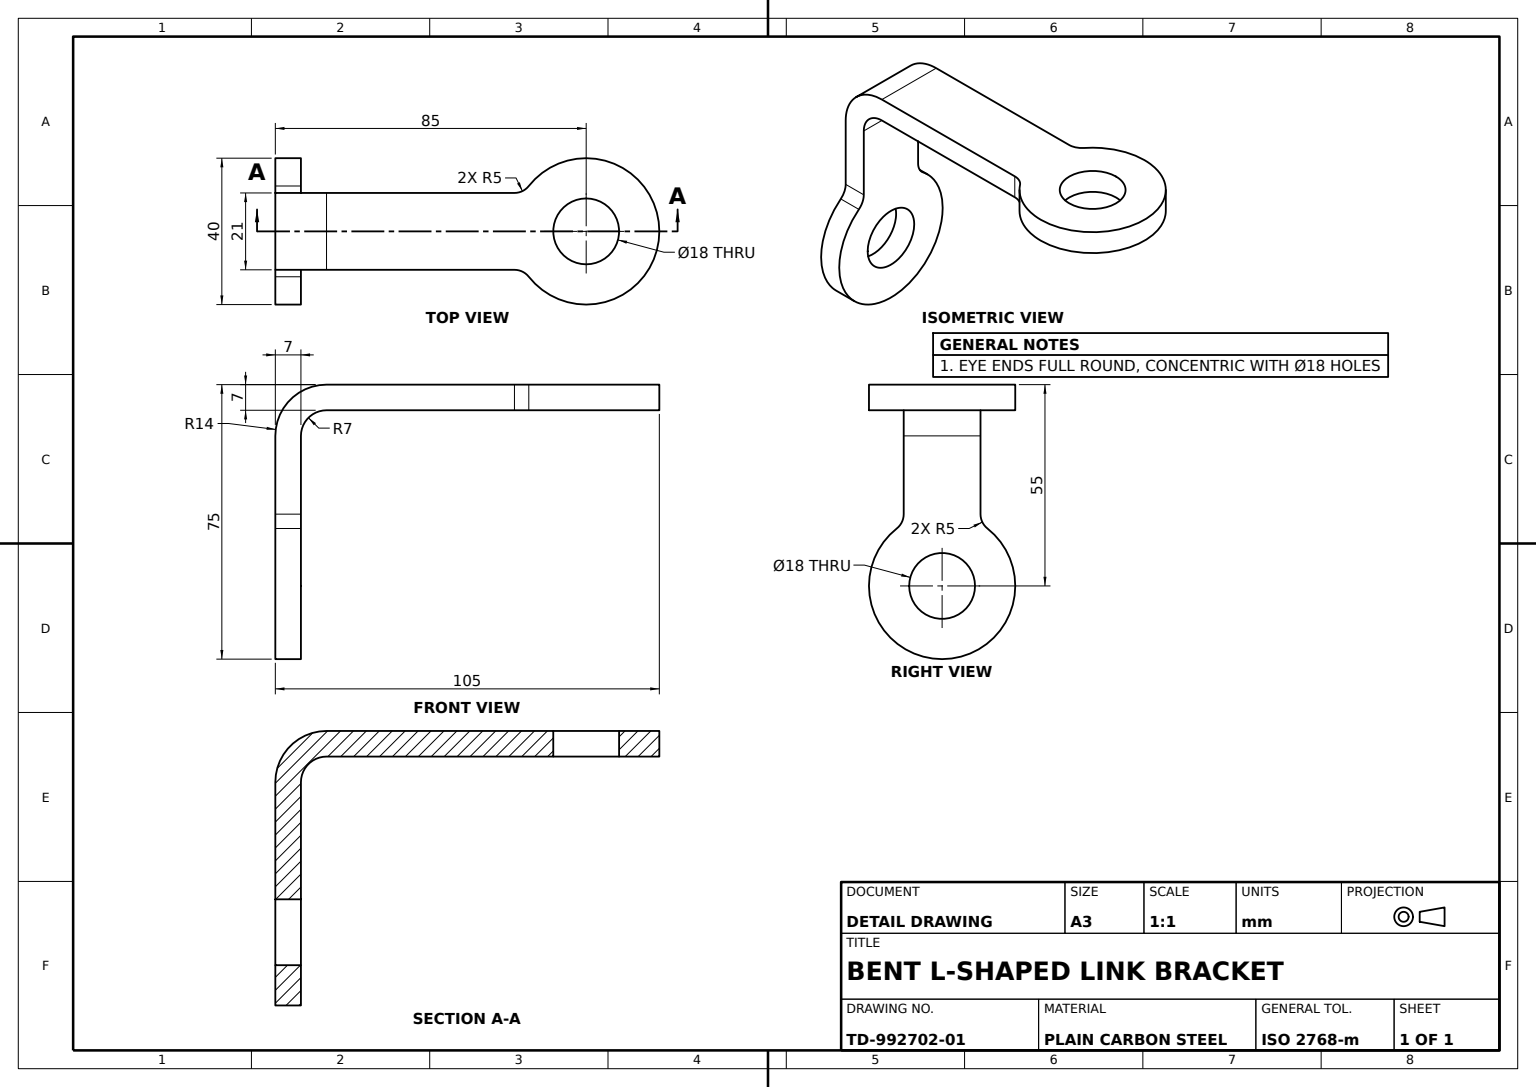
from build123d import *

# Parameters (mm, degrees)
HORIZONTAL_ARM_PROFILE_R    = 9
HORIZONTAL_ARM_7MM_DEPTH    = 7
VERTICAL_ARM_PROFILE_R      = 9
VERTICAL_ARM_7MM_DEPTH      = 7
BEND_FILLET_R5_R            = 5
HORIZONTAL_ARM_FILLET_R14_R = 14
BEND_FILLET_R7_R            = 7


with BuildPart() as part:
    # Horizontal Arm Profile → Horizontal Arm 7mm (new body)
    with BuildSketch(Plane(origin=(0, 0, 0), x_dir=(1, 0, 0), z_dir=(0, 1, 0))):
        with BuildLine():
            Line((-17.022044531, 10.5), (-85, 10.5))
            Line((-85, 10.5), (-85, -10.5))
            Line((-85, -10.5), (-17.022044531, -10.5))
            ThreePointArc((-17.022044531, -10.5), (20, 0), (-17.022044531, 10.5))
        make_face()
        with Locations(Location((0, 0, 0), (0, 0, 270))):
            Circle(HORIZONTAL_ARM_PROFILE_R, mode=Mode.SUBTRACT)
    extrude(amount=-HORIZONTAL_ARM_7MM_DEPTH)

    # Vertical Arm Profile → Vertical Arm 7mm (add)
    with BuildSketch(Plane(origin=(-85, 0, 0), x_dir=(0, 0, -1), z_dir=(1, 0, 0))):
        with BuildLine():
            Line((-10.5, 0), (-10.5, -37.977955469))
            ThreePointArc((-10.5, -37.977955469), (0, -75), (10.5, -37.977955469))
            Line((10.5, -37.977955469), (10.5, 0))
            Line((10.5, 0), (-10.5, 0))
        make_face()
        with Locations((0, -55)):
            Circle(VERTICAL_ARM_PROFILE_R, mode=Mode.SUBTRACT)
    extrude(amount=VERTICAL_ARM_7MM_DEPTH)

    # Bend Fillet R5
    bend_fillet_r5_edges = [part.edges().sort_by_distance(p)[0] for p in [
        (-81.5, -37.977955469, -10.5),
        (-81.5, -37.977955469, 10.5),
        (-17.022044531, -3.5, 10.5),
        (-17.022044531, -3.5, -10.5),
    ]]
    fillet(bend_fillet_r5_edges, radius=BEND_FILLET_R5_R)

    # Horizontal Arm Fillet R14
    horizontal_arm_fillet_r14_edges = [part.edges().sort_by_distance(p)[0] for p in [
        (-85, 0, 0),
    ]]
    fillet(horizontal_arm_fillet_r14_edges, radius=HORIZONTAL_ARM_FILLET_R14_R)

    # Bend Fillet R7
    bend_fillet_r7_edges = [part.edges().sort_by_distance(p)[0] for p in [
        (-78, -7, 0),
    ]]
    fillet(bend_fillet_r7_edges, radius=BEND_FILLET_R7_R)


solid = part.part
